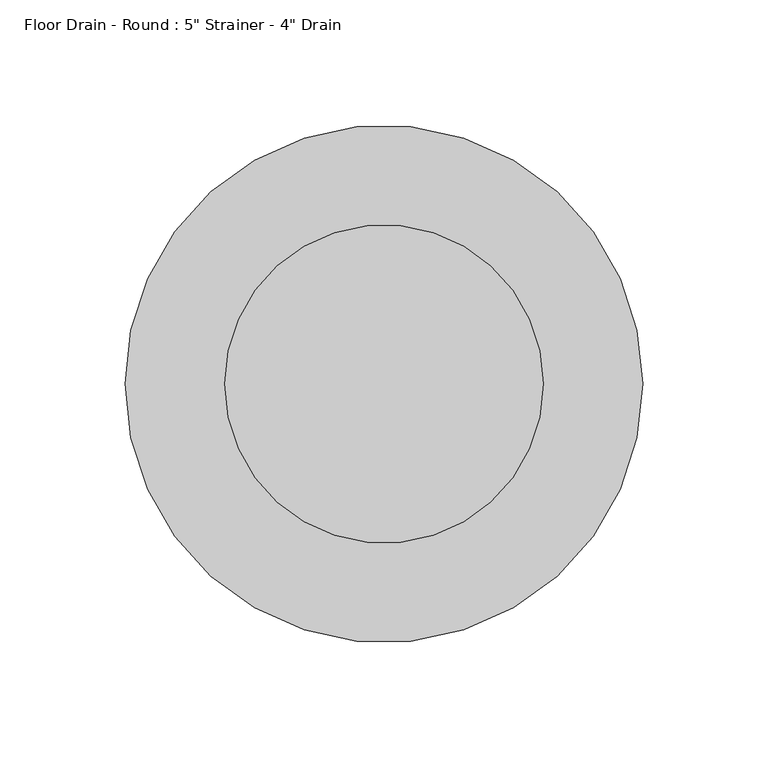
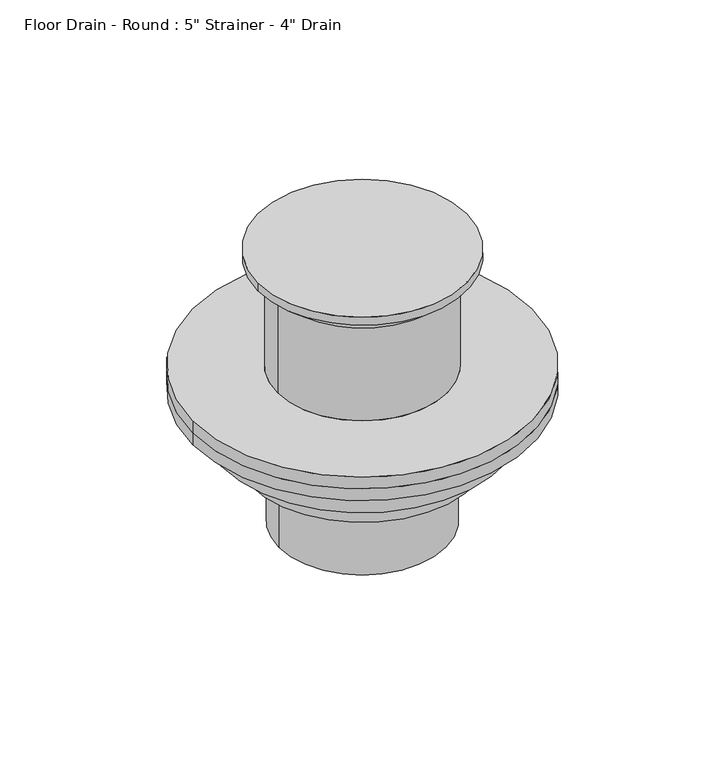
"""IFC4 building model written with IfcOpenShell, lengths in millimetres: flow terminal geometry."""

from ifc_helpers import new_model, si_unit, frame, origin, place, context, project, spatial, polyline, circle_curve, source, transform, mapped, element, save
from ifc_brep_helpers import plane_surface, cylinder_surface, revolved_surface, advanced_brep


def flow_terminal_5c41af1d(model_context):
    return source(origin(), model_context, "Body", "AdvancedBrep", [
        advanced_brep(
        [(103.1875, 0.0, -74.93), (-103.1875, 0.0, -74.93), (-51.59375, 0.0, -74.93), (51.59375, 0.0, -74.93), (103.1875, 0.0, -82.55), (-103.1875, 0.0, -82.55), (51.59375, 0.0, -15.24), (-51.59375, 0.0, -15.24), (-63.5, 0.0, -5.08), (63.5, 0.0, -5.08), (63.5, 0.0, 0.0), (-63.5, 0.0, 0.0)],
        [
            (0, 1, circle_curve(frame((0.0, 0.0, -74.93), z_axis=(0.0, 0.0, 1.0), x_axis=(-1.0, 0.0, 0.0)), 103.1875)),
            (1, 0, circle_curve(frame((0.0, 0.0, -74.93), z_axis=(0.0, 0.0, 1.0), x_axis=(-1.0, 0.0, 0.0)), 103.1875)),
            (2, 3, circle_curve(frame((0.0, 0.0, -74.93), z_axis=(0.0, 0.0, -1.0), x_axis=(-1.0, 0.0, 0.0)), 51.59375)),
            (3, 2, circle_curve(frame((0.0, 0.0, -74.93), z_axis=(0.0, 0.0, -1.0), x_axis=(-1.0, 0.0, 0.0)), 51.59375)),
            (4, 5, circle_curve(frame((0.0, 0.0, -82.55), z_axis=(0.0, 0.0, -1.0), x_axis=(-1.0, 0.0, 0.0)), 103.1875)),
            (5, 4, circle_curve(frame((0.0, 0.0, -82.55), z_axis=(0.0, 0.0, -1.0), x_axis=(-1.0, 0.0, 0.0)), 103.1875)),
            (0, 4),
            (5, 1),
            (6, 3),
            (2, 7),
            (7, 6, circle_curve(frame((0.0, 0.0, -15.24), z_axis=(0.0, 0.0, -1.0), x_axis=(-1.0, 0.0, 0.0)), 51.59375)),
            (6, 7, circle_curve(frame((0.0, 0.0, -15.24), z_axis=(0.0, 0.0, -1.0), x_axis=(-1.0, 0.0, 0.0)), 51.59375)),
            (7, 8),
            (8, 9, circle_curve(frame((0.0, 0.0, -5.08), z_axis=(0.0, 0.0, -1.0), x_axis=(-1.0, 0.0, 0.0)), 63.5)),
            (9, 6),
            (9, 8, circle_curve(frame((0.0, 0.0, -5.08), z_axis=(0.0, 0.0, -1.0), x_axis=(-1.0, 0.0, 0.0)), 63.5)),
            (10, 11, circle_curve(frame((0.0, 0.0, 0.0), z_axis=(0.0, 0.0, 1.0), x_axis=(-1.0, 0.0, 0.0)), 63.5)),
            (11, 10, circle_curve(frame((0.0, 0.0, 0.0), z_axis=(0.0, 0.0, 1.0), x_axis=(-1.0, 0.0, 0.0)), 63.5)),
            (10, 9),
            (8, 11),
        ],
        [
            plane_surface(frame((-103.1875, 0.0, -74.93), z_axis=(0.0, 0.0, 1.0), x_axis=(0.0, -1.0, 0.0))),
            plane_surface(frame((-103.1875, 0.0, -82.55), z_axis=(0.0, 0.0, -1.0), x_axis=(0.0, 1.0, 0.0))),
            cylinder_surface(frame((0.0, 0.0, -82.55), z_axis=(0.0, 0.0, 1.0), x_axis=(-1.0, 0.0, 0.0)), 103.1875),
            cylinder_surface(frame((0.0, 0.0, -74.93), z_axis=(0.0, 0.0, 1.0), x_axis=(-1.0, 0.0, 0.0)), 51.59375),
            revolved_surface(polyline([(-63.5, 0.0, -5.08), (-51.59375, 0.0, -15.24)]), (0.0, 0.0, 44.45), (0.0, 0.0, -1.0)),
            plane_surface(frame((-63.5, 0.0, 0.0), z_axis=(0.0, 0.0, 1.0), x_axis=(0.0, -1.0, 0.0))),
            cylinder_surface(frame((0.0, 0.0, -5.08), z_axis=(0.0, 0.0, 1.0), x_axis=(-1.0, 0.0, 0.0)), 63.5),
        ],
        [
            (0, [[1, 2], [3, 4]]),
            (1, [[5, 6]]),
            (2, [[-1, 7, -6, 8]]),
            (2, [[-2, -8, -5, -7]]),
            (3, [[9, -3, 10, 11]]),
            (3, [[-9, 12, -10, -4]]),
            (4, [[13, 14, 15, -11]]),
            (4, [[-13, -12, -15, 16]]),
            (5, [[17, 18]]),
            (6, [[-17, 19, -14, 20]]),
            (6, [[-18, -20, -16, -19]]),
        ],
    ),
        advanced_brep(
        [(50.8, 0.0, -174.625), (-50.8, 0.0, -174.625), (-50.8, 0.0, -128.5875), (50.8, 0.0, -128.5875), (68.2625, 0.0, -128.5875), (-68.2625, 0.0, -128.5875), (-68.2625, 0.0, -110.1725), (68.2625, 0.0, -110.1725), (85.725, 0.0, -110.1725), (-85.725, 0.0, -110.1725), (-85.725, 0.0, -90.17), (85.725, 0.0, -90.17), (103.1875, 0.0, -82.55), (-103.1875, 0.0, -82.55), (103.1875, 0.0, -90.17), (-103.1875, 0.0, -90.17)],
        [
            (0, 1, circle_curve(frame((0.0, 0.0, -174.625), z_axis=(0.0, 0.0, -1.0), x_axis=(-1.0, 0.0, 0.0)), 50.8)),
            (1, 0, circle_curve(frame((0.0, 0.0, -174.625), z_axis=(0.0, 0.0, -1.0), x_axis=(-1.0, 0.0, 0.0)), 50.8)),
            (1, 2),
            (2, 3, circle_curve(frame((0.0, 0.0, -128.5875), z_axis=(0.0, 0.0, -1.0), x_axis=(-1.0, 0.0, 0.0)), 50.8)),
            (3, 0),
            (3, 2, circle_curve(frame((0.0, 0.0, -128.5875), z_axis=(0.0, 0.0, -1.0), x_axis=(-1.0, 0.0, 0.0)), 50.8)),
            (4, 5, circle_curve(frame((0.0, 0.0, -128.5875), z_axis=(0.0, 0.0, -1.0), x_axis=(-1.0, 0.0, 0.0)), 68.2625)),
            (5, 4, circle_curve(frame((0.0, 0.0, -128.5875), z_axis=(0.0, 0.0, -1.0), x_axis=(-1.0, 0.0, 0.0)), 68.2625)),
            (5, 6),
            (6, 7, circle_curve(frame((0.0, 0.0, -110.1725), z_axis=(0.0, 0.0, -1.0), x_axis=(-1.0, 0.0, 0.0)), 68.2625)),
            (7, 4),
            (7, 6, circle_curve(frame((0.0, 0.0, -110.1725), z_axis=(0.0, 0.0, -1.0), x_axis=(-1.0, 0.0, 0.0)), 68.2625)),
            (8, 9, circle_curve(frame((0.0, 0.0, -110.1725), z_axis=(0.0, 0.0, -1.0), x_axis=(-1.0, 0.0, 0.0)), 85.725)),
            (9, 8, circle_curve(frame((0.0, 0.0, -110.1725), z_axis=(0.0, 0.0, -1.0), x_axis=(-1.0, 0.0, 0.0)), 85.725)),
            (9, 10),
            (10, 11, circle_curve(frame((0.0, 0.0, -90.17), z_axis=(0.0, 0.0, -1.0), x_axis=(-1.0, 0.0, 0.0)), 85.725)),
            (11, 8),
            (11, 10, circle_curve(frame((0.0, 0.0, -90.17), z_axis=(0.0, 0.0, -1.0), x_axis=(-1.0, 0.0, 0.0)), 85.725)),
            (12, 13, circle_curve(frame((0.0, 0.0, -82.55), z_axis=(0.0, 0.0, 1.0), x_axis=(-1.0, 0.0, 0.0)), 103.1875)),
            (13, 12, circle_curve(frame((0.0, 0.0, -82.55), z_axis=(0.0, 0.0, 1.0), x_axis=(-1.0, 0.0, 0.0)), 103.1875)),
            (14, 15, circle_curve(frame((0.0, 0.0, -90.17), z_axis=(0.0, 0.0, -1.0), x_axis=(-1.0, 0.0, 0.0)), 103.1875)),
            (15, 14, circle_curve(frame((0.0, 0.0, -90.17), z_axis=(0.0, 0.0, -1.0), x_axis=(-1.0, 0.0, 0.0)), 103.1875)),
            (12, 14),
            (15, 13),
        ],
        [
            plane_surface(frame((-50.8, 0.0, -174.625), z_axis=(0.0, 0.0, -1.0), x_axis=(0.0, 1.0, 0.0))),
            cylinder_surface(frame((0.0, 0.0, -174.625), z_axis=(0.0, 0.0, 1.0), x_axis=(-1.0, 0.0, 0.0)), 50.8),
            plane_surface(frame((-68.2625, 0.0, -128.5875), z_axis=(0.0, 0.0, -1.0), x_axis=(0.0, 1.0, 0.0))),
            cylinder_surface(frame((0.0, 0.0, -128.5875), z_axis=(0.0, 0.0, 1.0), x_axis=(-1.0, 0.0, 0.0)), 68.2625),
            plane_surface(frame((-85.725, 0.0, -110.1725), z_axis=(0.0, 0.0, -1.0), x_axis=(0.0, 1.0, 0.0))),
            cylinder_surface(frame((0.0, 0.0, -110.1725), z_axis=(0.0, 0.0, 1.0), x_axis=(-1.0, 0.0, 0.0)), 85.725),
            plane_surface(frame((-103.1875, 0.0, -82.55), z_axis=(0.0, 0.0, 1.0), x_axis=(0.0, -1.0, 0.0))),
            plane_surface(frame((-103.1875, 0.0, -90.17), z_axis=(0.0, 0.0, -1.0), x_axis=(0.0, 1.0, 0.0))),
            cylinder_surface(frame((0.0, 0.0, -90.17), z_axis=(0.0, 0.0, 1.0), x_axis=(-1.0, 0.0, 0.0)), 103.1875),
        ],
        [
            (0, [[1, 2]]),
            (1, [[-2, 3, 4, 5]]),
            (1, [[-1, -5, 6, -3]]),
            (2, [[7, 8], [-4, -6]]),
            (3, [[-8, 9, 10, 11]]),
            (3, [[-7, -11, 12, -9]]),
            (4, [[13, 14], [-10, -12]]),
            (5, [[-14, 15, 16, 17]]),
            (5, [[-13, -17, 18, -15]]),
            (6, [[19, 20]]),
            (7, [[21, 22], [-16, -18]]),
            (8, [[-19, 23, -22, 24]]),
            (8, [[-20, -24, -21, -23]]),
        ],
    ),
    ])


if __name__ == "__main__":
    model = new_model("IFC4")
    model_context = context("Model", 3, world=origin())
    ifc_project = project(units=[si_unit("LENGTHUNIT", "METRE", prefix="MILLI")], contexts=[model_context])
    site = spatial("IfcSite", under=ifc_project)
    building = spatial("IfcBuilding", under=site)
    placement = place(None, origin())
    flow_terminal_shape = flow_terminal_5c41af1d(model_context)
    element("IfcFlowTerminal", 1, ObjectType="Floor Drain - Round : 5\" Strainer - 4\" Drain", at=placement, inside=building, context=model_context, shape_type="MappedRepresentation", body=[
        mapped(flow_terminal_shape, transform((0.0, 0.0, 0.0), x_axis=(1.0, 0.0, 0.0), y_axis=(0.0, 1.0, 0.0), z_axis=(0.0, 0.0, 1.0))),
    ])
    save(model, "model.ifc")

# Revit data of these elements
# Type "Floor Drain - Round : 5\" Strainer - 4\" Drain"
#   WFU = 4
#   Strainer Height = 0' - 3 1/4"
#   Strainer Radius = 0' - 2 1/2"
#   Strainer Diameter = 0' - 5"
#   Radius 6 = 0' - 0 5/8"
#   Radius 5 = 0' - 1 1/4"
#   Radius 4 = 0' - 1 7/8"
#   Radius 2 = 0' - 3 3/8"
#   Radius 1 = 0' - 2 11/16"
#   Radius 3 = 0' - 2 1/32"
#   Pipe Radius = 2"
#   Pipe Diameter = 4"
#   Height 2 = 0' - 0.725"
#   Height 1 = 0' - 1 13/16"
#   Body Radius = 0' - 4 1/16"
#   Body Height = 0' - 3 5/8"
#   Body Diameter = 0' - 8 1/8"
#   Drain Material = none
#   HWFU = 0
#   Default Elevation = 0
#   CWFU = 0
